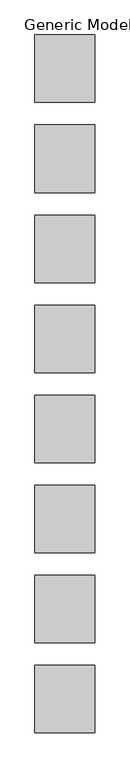
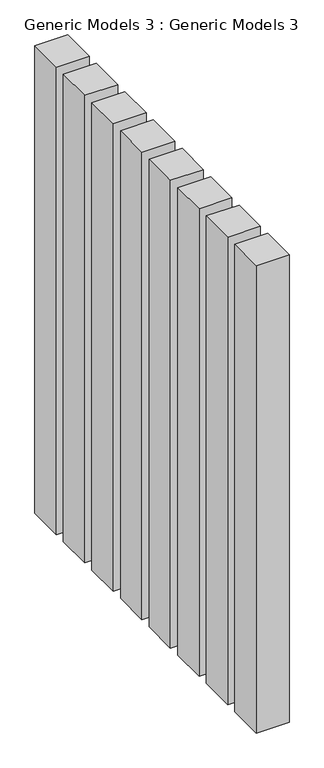
"""IFC4 building model written with IfcOpenShell, lengths in millimetres: proxy geometry, Generic Models 3 : Generic Models 3."""

from ifc_helpers import new_model, si_unit, frame, origin, place, context, project, spatial, polyline, outline, extrude, source, transform, mapped, element, save


def generic_models_3_generic_models_3_71021abf(model_context):
    return source(origin(), model_context, "Body", "SweptSolid", [
        extrude(outline(polyline([(-2052.5656154, 966.7378753), (-2255.7656154, 966.7378753), (-2255.7656154, 1195.3378753), (-2052.5656154, 1195.3378753), (-2052.5656154, 966.7378753)])), frame((0.0, 0.0, 3048.0), z_axis=(0.0, 0.0, 1.0), x_axis=(1.0, 0.0, 0.0)), (0.0, 0.0, 1.0), 3048.0),
        extrude(outline(polyline([(-2052.5656154, 1271.5378753), (-2255.7656154, 1271.5378753), (-2255.7656154, 1500.1378753), (-2052.5656154, 1500.1378753), (-2052.5656154, 1271.5378753)])), frame((0.0, 0.0, 3048.0), z_axis=(0.0, 0.0, 1.0), x_axis=(1.0, 0.0, 0.0)), (0.0, 0.0, 1.0), 3048.0),
        extrude(outline(polyline([(-2052.5656154, 1576.3378753), (-2255.7656154, 1576.3378753), (-2255.7656154, 1804.9378753), (-2052.5656154, 1804.9378753), (-2052.5656154, 1576.3378753)])), frame((0.0, 0.0, 3048.0), z_axis=(0.0, 0.0, 1.0), x_axis=(1.0, 0.0, 0.0)), (0.0, 0.0, 1.0), 3048.0),
        extrude(outline(polyline([(-2052.5656154, 1881.1378753), (-2255.7656154, 1881.1378753), (-2255.7656154, 2109.7378753), (-2052.5656154, 2109.7378753), (-2052.5656154, 1881.1378753)])), frame((0.0, 0.0, 3048.0), z_axis=(0.0, 0.0, 1.0), x_axis=(1.0, 0.0, 0.0)), (0.0, 0.0, 1.0), 3048.0),
        extrude(outline(polyline([(-2052.5656154, 2185.9378753), (-2255.7656154, 2185.9378753), (-2255.7656154, 2414.5378753), (-2052.5656154, 2414.5378753), (-2052.5656154, 2185.9378753)])), frame((0.0, 0.0, 3048.0), z_axis=(0.0, 0.0, 1.0), x_axis=(1.0, 0.0, 0.0)), (0.0, 0.0, 1.0), 3048.0),
        extrude(outline(polyline([(-2052.5656154, 2490.7378753), (-2255.7656154, 2490.7378753), (-2255.7656154, 2719.3378753), (-2052.5656154, 2719.3378753), (-2052.5656154, 2490.7378753)])), frame((0.0, 0.0, 3048.0), z_axis=(0.0, 0.0, 1.0), x_axis=(1.0, 0.0, 0.0)), (0.0, 0.0, 1.0), 3048.0),
        extrude(outline(polyline([(-2052.5656154, 2795.5378753), (-2255.7656154, 2795.5378753), (-2255.7656154, 3024.1378753), (-2052.5656154, 3024.1378753), (-2052.5656154, 2795.5378753)])), frame((0.0, 0.0, 3048.0), z_axis=(0.0, 0.0, 1.0), x_axis=(1.0, 0.0, 0.0)), (0.0, 0.0, 1.0), 3048.0),
        extrude(outline(polyline([(-2052.5656154, 3100.3378753), (-2255.7656154, 3100.3378753), (-2255.7656154, 3328.9378753), (-2052.5656154, 3328.9378753), (-2052.5656154, 3100.3378753)])), frame((0.0, 0.0, 3048.0), z_axis=(0.0, 0.0, 1.0), x_axis=(1.0, 0.0, 0.0)), (0.0, 0.0, 1.0), 3048.0),
    ])


if __name__ == "__main__":
    model = new_model("IFC4")
    model_context = context("Model", 3, world=origin())
    ifc_project = project(units=[si_unit("LENGTHUNIT", "METRE", prefix="MILLI")], contexts=[model_context])
    site = spatial("IfcSite", under=ifc_project)
    building = spatial("IfcBuilding", under=site)
    placement = place(None, origin())
    generic_models_3_generic_models_3_shape = generic_models_3_generic_models_3_71021abf(model_context)
    element("IfcBuildingElementProxy", 1, Name="Generic Models 3 : Generic Models 3", ObjectType="Generic Models 3 : Generic Models 3", at=placement, inside=building, context=model_context, shape_type="MappedRepresentation", body=[
        mapped(generic_models_3_generic_models_3_shape, transform((0.0, 0.0, 0.0), x_axis=(1.0, 0.0, 0.0), y_axis=(0.0, 1.0, 0.0), z_axis=(0.0, 0.0, 1.0))),
    ])
    save(model, "model.ifc")

# Revit data of these elements
# Element 1 (IfcBuildingElementProxy, "Generic Models 3 : Generic Models 3")
#   Materials on its faces: "LIGHT BEIGE"
# Materials
#   "LIGHT BEIGE": class "Generic", colour RGB 120 120 120, transparency 0, Cost = 0
